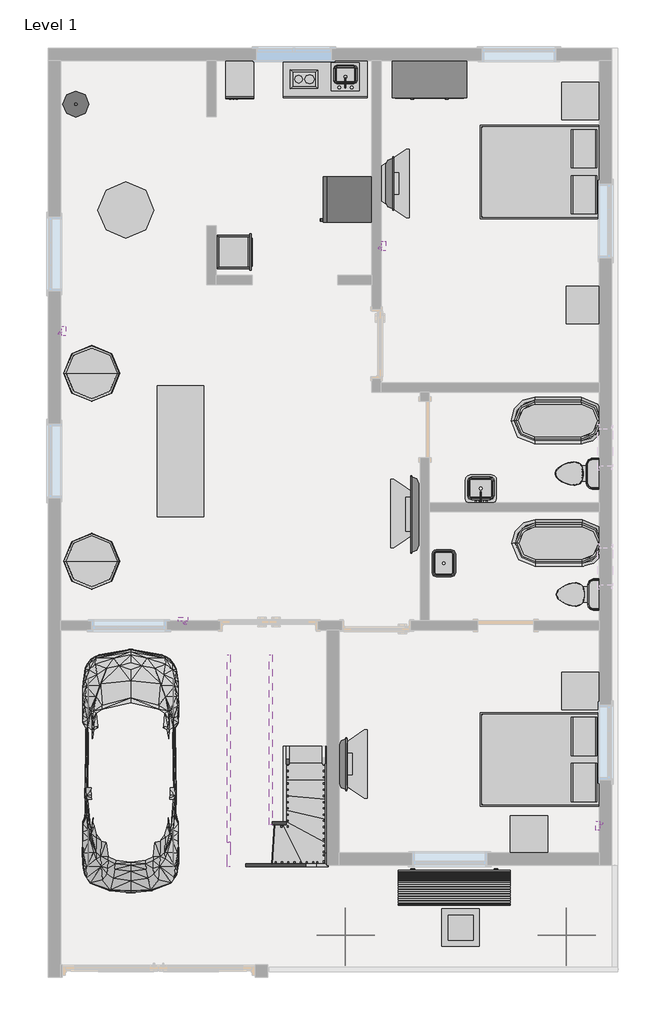
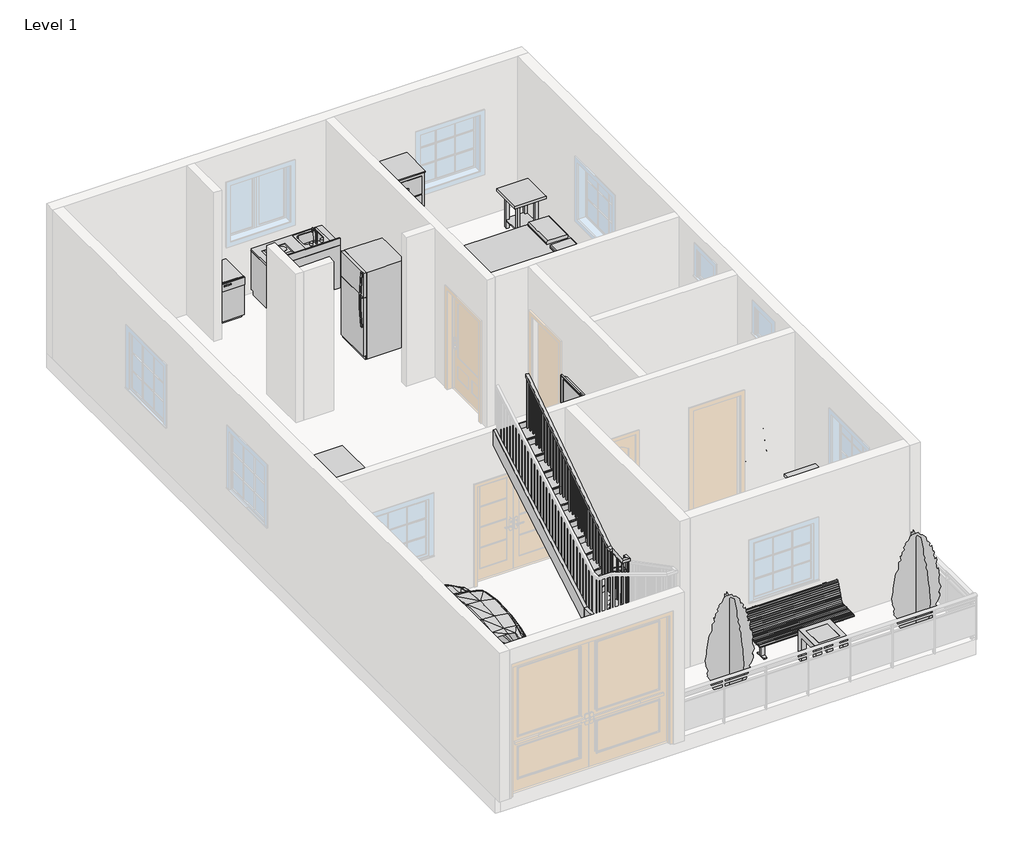
# One storey, part 3 of 3: 19 furniture elements, 10 proxies, 9 members, 8 flow terminals, 3 geographic elements, 1 railing, 1 stair flight.
# Revit data of these elements (continued)
# Materials (continued)
#   "Steel, Chrome Plated": class "Metal", colour RGB 17 17 17, transparency 0, Description = "Chromiuim plated steel", Cost = 0
#   "Steel, Polished": class "Metal", colour RGB 57 57 57, transparency 0, Description = "Polished steel", Cost = 0
#   "Cabinets": colour RGB 249 249 249, transparency 0
#   "Cabinets - Handles": class "Metal", colour RGB 57 57 57, transparency 0
#   "Metal - Stainless Steel, Polished": class "Metal", colour RGB 216 216 216, transparency 0
#   "Steel, Paint Finish, Ivory, Glossy": class "Metal", colour RGB 247 247 239, transparency 0, Description = "Steel, paint finish, ivory, glossy", Cost = 0
#   "Porcelain, Linen": class "Ceramic", colour RGB 249 239 230, transparency 0, Description = "Porcelain, linen", Cost = 0
#   "Laminate, Linen, Matte": class "Plastic", colour RGB 249 239 230, transparency 0, Description = "Plastic Laminate - Linen, Matte", Cost = 0
#   "Porcelain, Ivory": class "Ceramic", colour RGB 247 247 239, transparency 0, Description = "Porcelain, ivory", Cost = 0
#   "Birch": class "Wood", colour RGB 224 178 126, transparency 0, Description = "Betula Alleghaniensis", Cost = 0
#   "Linen, White": class "Textile", colour RGB 247 247 239, transparency 0, Description = "Linen, white", Cost = 0
#   "Laminate - Ivory, Glossy": colour RGB 247 247 239, transparency 0
#   "Laminate, Ivory, Matte": class "Plastic", colour RGB 247 247 239, transparency 0, Description = "Plastic Laminate - Ivory, Matte", Cost = 0
#   "Cherry": class "Wood", colour RGB 226 177 128, transparency 0, Description = "Prunus Serotina", Cost = 0
#   "Melamine - Gray": class "Wood", colour RGB 49 49 49, transparency 0
#   "Glass - Clear, Grey": class "Glass", colour RGB 252 255 255, transparency 0.64
#   "Pine": class "Wood", colour RGB 223 192 134, transparency 0, Description = "Pinus Echinata", Cost = 0
#   "Wood - Teak": class "Wood", colour RGB 120 73 19, transparency 0
#   "Steel, Paint Finish, Dark Gray, Matte": class "Metal", colour RGB 98 98 98, transparency 0, Description = "Steel, paint finish, dark gray, matte", Cost = 0
#   "Steel": class "Metal", colour RGB 247 247 247, transparency 0, Description = "Steel, mill finish", Cost = 0
#   "Glass": class "Glass", colour RGB 0 128 192, transparency 0.75, Description = "Soda Lime Glass", Cost = 0
#   "Counter Top": class "Wood", colour RGB 226 177 128, transparency 0
#   "TV - Black": colour RGB 49 49 49, transparency 0
#   "TV - Glass": colour RGB 157 157 157, transparency 0.9
#   "TV - Screen": colour RGB 0 0 0, transparency 0
#   "Glass - Shelves": class "Glass", colour RGB 167 167 167, transparency 0.9
